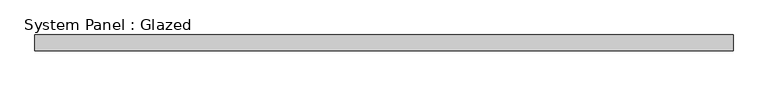
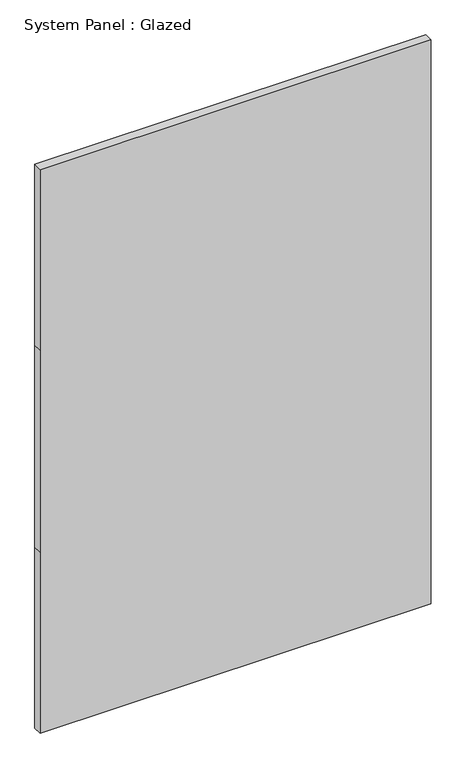
"""IFC4 building model written with IfcOpenShell, lengths in millimetres: plate geometry, System Panel : Glazed."""

from ifc_helpers import new_model, si_unit, frame, origin, place, context, project, spatial, polyline, outline, extrude, source, transform, mapped, element, save


def system_panel_glazed_a9ff3cf1(model_context):
    return source(origin(), model_context, "Body", "SweptSolid", [
        extrude(outline(polyline([(0.0, -561.975), (0.0, 561.975), (549.2937999, 561.975), (1162.0875999, 561.975), (1711.3813998, 561.975), (1711.3813998, -561.975), (1162.0875999, -561.975), (549.2937999, -561.975), (0.0, -561.975)])), frame((0.0, 19.05, 0.0), z_axis=(0.0, 1.0, 0.0), x_axis=(0.0, 0.0, 1.0)), (0.0, 0.0, 1.0), 25.4),
    ])


if __name__ == "__main__":
    model = new_model("IFC4")
    model_context = context("Model", 3, world=origin())
    ifc_project = project(units=[si_unit("LENGTHUNIT", "METRE", prefix="MILLI")], contexts=[model_context])
    site = spatial("IfcSite", under=ifc_project)
    building = spatial("IfcBuilding", under=site)
    placement = place(None, origin())
    system_panel_glazed_shape = system_panel_glazed_a9ff3cf1(model_context)
    element("IfcPlate", 1, ObjectType="System Panel : Glazed", at=placement, inside=building, context=model_context, shape_type="MappedRepresentation", body=[
        mapped(system_panel_glazed_shape, transform((0.0, 0.0, 0.0), x_axis=(1.0, 0.0, 0.0), y_axis=(0.0, 1.0, 0.0), z_axis=(0.0, 0.0, 1.0))),
    ])
    save(model, "model.ifc")

# Revit data of these elements
# Type "System Panel : Glazed"
#   Construction Type Id = "GSP4R"
#   Analytic Construction = "1/8 in Pilkington single glazing"
#   Visual Light Transmittance = 0.9
#   Solar Heat Gain Coefficient = 0.86
#   Heat Transfer Coefficient (U) = 1.18115 BTU/(h·ft²·°F)
#   Define Thermal Properties by = 1
# Element 1 (IfcPlate, "System Panel : Glazed")
#   Materials on its faces: "Glass"
# Materials
#   "Glass": class "Glass", colour RGB 0 128 192, transparency 0.75, Description = "Soda Lime Glass", Cost = 0
